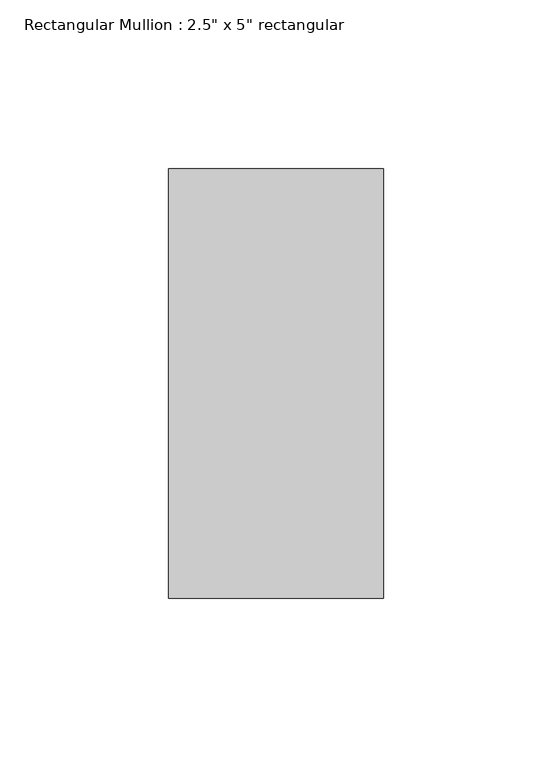
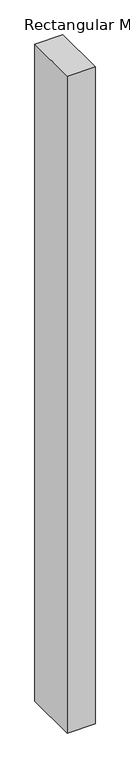
"""IFC4 building model written with IfcOpenShell, lengths in millimetres: member geometry."""

from ifc_helpers import new_model, si_unit, frame, origin, place, context, project, spatial, polyline, outline, extrude, source, transform, mapped, element, save


def member_247435d8(model_context):
    return source(origin(), model_context, "Body", "SweptSolid", [
        extrude(outline(polyline([(0.0, 63.5), (0.0, -63.5), (-63.5, -63.5), (-63.5, 63.5), (0.0, 63.5)])), frame((0.0, 0.0, -1581.15), z_axis=(0.0, 0.0, 1.0), x_axis=(1.0, 0.0, 0.0)), (0.0, 0.0, 1.0), 1581.15),
    ])


if __name__ == "__main__":
    model = new_model("IFC4")
    model_context = context("Model", 3, world=origin())
    ifc_project = project(units=[si_unit("LENGTHUNIT", "METRE", prefix="MILLI")], contexts=[model_context])
    site = spatial("IfcSite", under=ifc_project)
    building = spatial("IfcBuilding", under=site)
    placement = place(None, origin())
    member_shape = member_247435d8(model_context)
    element("IfcMember", 1, ObjectType="Rectangular Mullion : 2.5\" x 5\" rectangular", at=placement, inside=building, context=model_context, shape_type="MappedRepresentation", body=[
        mapped(member_shape, transform((0.0, 0.0, 0.0), x_axis=(1.0, 0.0, 0.0), y_axis=(0.0, 1.0, 0.0), z_axis=(0.0, 0.0, 1.0))),
    ])
    save(model, "model.ifc")

# Revit data of these elements
# Type "Rectangular Mullion : 2.5\" x 5\" rectangular"
#   built-in parameter 1007304 = 0.416667 (stored number, unit not read)
#   built-in parameter 1007301 = 0.104167 (stored number, unit not read)
#   built-in parameter 1007300 = 0.104167 (stored number, unit not read)
# Element 1 (IfcMember, "Rectangular Mullion : 2.5\" x 5\" rectangular")
#   Materials on its faces: "Aluminum"
# Materials
#   "Aluminum": class "Metal", colour RGB 247 247 247, transparency 0, Description = "Aluminum 6061", Cost = 0
